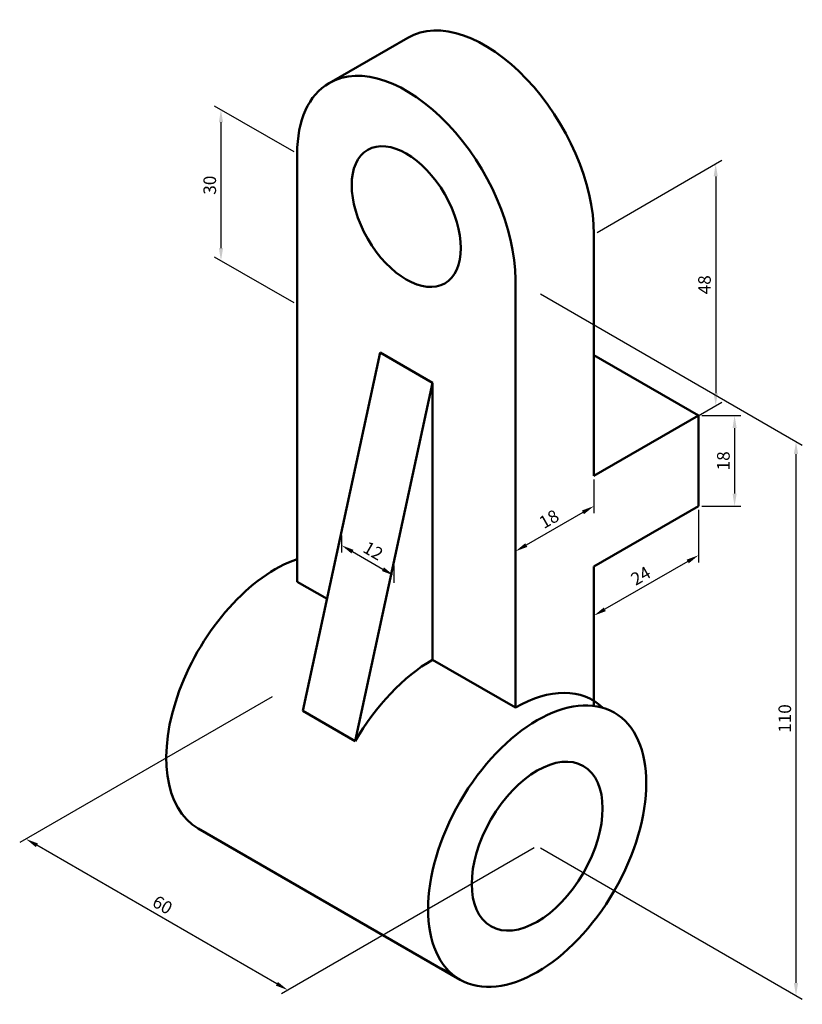
# Model space of a CAD drawing. Units: millimetres. Extents: x 3133 to 3289, y 1000 to 1195.
import ezdxf

# ---------------------------------------------------------------- set-up
doc = ezdxf.new("R2010")
doc.units = ezdxf.units.MM
doc.layers.add('M-DIMS', color=2, linetype='Continuous', lineweight=25)
doc.layers.add('M-OUTL', color=7, linetype='Continuous', lineweight=50)
doc.styles.get("Standard").update_dxf_attribs({"font": 'arial.ttf'})
doc.dimstyles.new('ISO-25', dxfattribs={"dimtxt": 2.5, "dimasz": 2.5, "dimexe": 1.25, "dimexo": 0.625, "dimtad": 1, "dimtxsty": 'Standard', "dimcen": 2.5, "dimadec": 0, "dimazin": 0, "dimtfac": 1, "dimtmove": 0, "dimatfit": 3, "dimfxl": 1, "dimarcsym": 0})

# ---------------------------------------------------------------- blocks, each defined once
blk = doc.blocks.new('*D1')
at = {"layer": 'Defpoints', "color": 0, "transparency": 16777216}
for p in [(3247.42, 1152.8), (3271.59, 1118.76), (3247.42, 1104.8)]:
    blk.add_point(p, dxfattribs=at)
at = {"layer": 'M-DIMS', "color": 0, "lineweight": -2, "transparency": 16777216}
for p, q in [((3248.04, 1153.16), (3272.84, 1167.48)), ((3271.59, 1164.26), (3271.59, 1121.26)), ((3248.04, 1105.16), (3272.84, 1119.48))]:
    blk.add_line(p, q, dxfattribs=at)
at = {"layer": 'M-DIMS', "color": 0, "transparency": 16777216}
for points in [[(3271.18, 1164.26), (3272.01, 1164.26), (3271.59, 1166.76)], [(3271.18, 1121.26), (3272.01, 1121.26), (3271.59, 1118.76)]]:
    blk.add_solid(points, dxfattribs=at)
at = {"layer": 'M-DIMS', "color": 0, "transparency": 16777216, "insert": (3269.69, 1142.76), "char_height": 2.5, "attachment_point": 5, "rotation": 90}
blk.add_mtext('48', dxfattribs=at)
blk = doc.blocks.new('*D2')
at = {"layer": 'Defpoints', "color": 0, "transparency": 16777216}
for p in [(3268.2, 1116.8), (3268.2, 1098.8), (3275.34, 1098.8)]:
    blk.add_point(p, dxfattribs=at)
at = {"layer": 'M-DIMS', "color": 0, "lineweight": -2, "transparency": 16777216}
for p, q in [((3268.83, 1116.8), (3276.59, 1116.8)), ((3275.34, 1114.3), (3275.34, 1101.3)), ((3268.83, 1098.8), (3276.59, 1098.8))]:
    blk.add_line(p, q, dxfattribs=at)
at = {"layer": 'M-DIMS', "color": 0, "transparency": 16777216}
for points in [[(3274.93, 1114.3), (3275.76, 1114.3), (3275.34, 1116.8)], [(3274.93, 1101.3), (3275.76, 1101.3), (3275.34, 1098.8)]]:
    blk.add_solid(points, dxfattribs=at)
at = {"layer": 'M-DIMS', "color": 0, "transparency": 16777216, "insert": (3273.44, 1107.8), "char_height": 2.5, "attachment_point": 5, "rotation": 90}
blk.add_mtext('18', dxfattribs=at)
blk = doc.blocks.new('*D3')
at = {"layer": 'Defpoints', "color": 0, "transparency": 16777216}
for p in [(3268.2, 1098.8), (3247.42, 1086.8), (3247.42, 1077.07)]:
    blk.add_point(p, dxfattribs=at)
at = {"layer": 'M-DIMS', "color": 0, "lineweight": -2, "transparency": 16777216}
for p, q in [((3268.2, 1098.08), (3268.2, 1087.62)), ((3266.04, 1087.82), (3249.58, 1078.32)), ((3247.42, 1086.08), (3247.42, 1075.62))]:
    blk.add_line(p, q, dxfattribs=at)
at = {"layer": 'M-DIMS', "color": 0, "transparency": 16777216}
for points in [[(3265.83, 1088.18), (3266.25, 1087.46), (3268.2, 1089.07)], [(3249.38, 1078.68), (3249.79, 1077.96), (3247.42, 1077.07)]]:
    blk.add_solid(points, dxfattribs=at)
at = {"layer": 'M-DIMS', "color": 0, "transparency": 16777216, "insert": (3256.87, 1084.7), "char_height": 2.5, "attachment_point": 5, "rotation": 30}
blk.add_mtext('24', dxfattribs=at)
blk = doc.blocks.new('*D4')
at = {"layer": 'Defpoints', "color": 0, "transparency": 16777216}
for p in [(3188.53, 1168.8), (3173.4, 1147.53), (3188.53, 1138.8)]:
    blk.add_point(p, dxfattribs=at)
at = {"layer": 'M-DIMS', "color": 0, "lineweight": -2, "transparency": 16777216}
for p, q in [((3187.9, 1169.16), (3172.15, 1178.25)), ((3173.4, 1175.03), (3173.4, 1150.03)), ((3187.9, 1139.16), (3172.15, 1148.25))]:
    blk.add_line(p, q, dxfattribs=at)
at = {"layer": 'M-DIMS', "color": 0, "transparency": 16777216}
for points in [[(3172.98, 1175.03), (3173.82, 1175.03), (3173.4, 1177.53)], [(3172.98, 1150.03), (3173.82, 1150.03), (3173.4, 1147.53)]]:
    blk.add_solid(points, dxfattribs=at)
at = {"layer": 'M-DIMS', "color": 0, "transparency": 16777216, "insert": (3171.5, 1162.53), "char_height": 2.5, "attachment_point": 5, "rotation": 90}
blk.add_mtext('30', dxfattribs=at)
blk = doc.blocks.new('*D5')
at = {"layer": 'Defpoints', "color": 0, "transparency": 16777216}
for p in [(3184.2, 1061.3), (3134.71, 1032.72), (3236.16, 1031.3)]:
    blk.add_point(p, dxfattribs=at)
at = {"layer": 'M-DIMS', "color": 0, "lineweight": -2, "transparency": 16777216}
for p, q in [((3183.57, 1060.94), (3133.46, 1032)), ((3184.5, 1003.97), (3136.87, 1031.47)), ((3235.54, 1030.94), (3185.42, 1002))]:
    blk.add_line(p, q, dxfattribs=at)
at = {"layer": 'M-DIMS', "color": 0, "transparency": 16777216}
for points in [[(3137.08, 1031.83), (3136.66, 1031.11), (3134.71, 1032.72)], [(3184.71, 1004.33), (3184.3, 1003.61), (3186.67, 1002.72)]]:
    blk.add_solid(points, dxfattribs=at)
at = {"layer": 'M-DIMS', "color": 0, "transparency": 16777216, "insert": (3161.64, 1019.37), "char_height": 2.5, "attachment_point": 5, "rotation": 330}
blk.add_mtext('60', dxfattribs=at)
blk = doc.blocks.new('*D6')
at = {"layer": 'Defpoints', "color": 0, "transparency": 16777216}
for p in [(3236.16, 1141.3), (3287.53, 1111.64), (3236.16, 1031.3)]:
    blk.add_point(p, dxfattribs=at)
at = {"layer": 'M-DIMS', "color": 0, "lineweight": -2, "transparency": 16777216}
for p, q in [((3236.79, 1140.94), (3288.78, 1110.92)), ((3287.53, 1004.14), (3287.53, 1109.14)), ((3236.79, 1030.94), (3288.78, 1000.92))]:
    blk.add_line(p, q, dxfattribs=at)
at = {"layer": 'M-DIMS', "color": 0, "transparency": 16777216}
for points in [[(3287.11, 1109.14), (3287.95, 1109.14), (3287.53, 1111.64)], [(3287.11, 1004.14), (3287.95, 1004.14), (3287.53, 1001.64)]]:
    blk.add_solid(points, dxfattribs=at)
at = {"layer": 'M-DIMS', "color": 0, "transparency": 16777216, "insert": (3285.63, 1056.64), "char_height": 2.5, "attachment_point": 5, "rotation": 90}
blk.add_mtext('110', dxfattribs=at)
blk = doc.blocks.new('*D7')
at = {"layer": 'Defpoints', "color": 0, "transparency": 16777216}
for p in [(3197.33, 1093.72), (3207.72, 1087.72), (3207.72, 1085.03)]:
    blk.add_point(p, dxfattribs=at)
at = {"layer": 'M-DIMS', "color": 0, "lineweight": -2, "transparency": 16777216}
for p, q in [((3197.33, 1093), (3197.33, 1089.58)), ((3199.49, 1089.78), (3205.56, 1086.28)), ((3207.72, 1087), (3207.72, 1083.58))]:
    blk.add_line(p, q, dxfattribs=at)
at = {"layer": 'M-DIMS', "color": 0, "transparency": 16777216}
for points in [[(3199.7, 1090.14), (3199.29, 1089.42), (3197.33, 1091.03)], [(3205.76, 1086.64), (3205.35, 1085.92), (3207.72, 1085.03)]]:
    blk.add_solid(points, dxfattribs=at)
at = {"layer": 'M-DIMS', "color": 0, "transparency": 16777216, "insert": (3203.46, 1089.66), "char_height": 2.5, "attachment_point": 5, "rotation": 330}
blk.add_mtext('12', dxfattribs=at)
blk = doc.blocks.new('*D8')
at = {"layer": 'Defpoints', "color": 0, "transparency": 16777216}
for p in [(3247.42, 1104.8), (3231.83, 1095.8), (3231.83, 1089.83)]:
    blk.add_point(p, dxfattribs=at)
at = {"layer": 'M-DIMS', "color": 0, "lineweight": -2, "transparency": 16777216}
for p, q in [((3247.42, 1104.08), (3247.42, 1097.38)), ((3245.25, 1097.57), (3233.99, 1091.08)), ((3231.83, 1095.08), (3231.83, 1088.38))]:
    blk.add_line(p, q, dxfattribs=at)
at = {"layer": 'M-DIMS', "color": 0, "transparency": 16777216}
for points in [[(3245.04, 1097.94), (3245.46, 1097.21), (3247.42, 1098.82)], [(3233.79, 1091.44), (3234.2, 1090.71), (3231.83, 1089.83)]]:
    blk.add_solid(points, dxfattribs=at)
at = {"layer": 'M-DIMS', "color": 0, "transparency": 16777216, "insert": (3238.67, 1095.97), "char_height": 2.5, "attachment_point": 5, "rotation": 29.9986}
blk.add_mtext('18', dxfattribs=at)

msp = doc.modelspace()

# ---------------------------------------------------------------- linework, layer by layer
at = {"layer": 'M-OUTL'}
for p, q in [((3210.458, 1191.814), (3194.87, 1182.814)), ((3188.529, 1168.798), (3188.529, 1083.798)), ((3247.418, 1152.798), (3247.418, 1104.798)), ((3231.83, 1143.798), (3231.83, 1058.798)), ((3189.674, 1058.136), (3204.983, 1129.298)), ((3215.375, 1123.298), (3204.983, 1129.298)), ((3268.203, 1116.798), (3247.418, 1128.798)), ((3215.375, 1123.298), (3200.066, 1052.136)), ((3215.375, 1123.298), (3215.375, 1068.298)), ((3247.418, 1104.798), (3268.203, 1116.798)), ((3268.203, 1116.798), (3268.203, 1098.798)), ((3268.203, 1098.798), (3247.418, 1086.798)), ((3247.418, 1086.798), (3247.418, 1059.152)), ((3194.458, 1080.374), (3188.529, 1083.798)), ((3215.375, 1068.298), (3231.83, 1058.798)), ((3200.066, 1052.136), (3189.674, 1058.136)), ((3168.889, 1034.781), (3220.851, 1004.781))]:
    msp.add_line(p, q, dxfattribs=at)
for centre, major_axis, start_param, end_param in [((3225.768, 1165.298), (15.309, -26.517), 7.0685835, 9.424778), ((3210.179, 1156.298), (15.309, -26.517), 0.7853982, 3.1415927), ((3210.179, 1156.298), (15.309, -26.517), 3.1415927, 3.9269908), ((3184.199, 1061.298), (-15.309, -26.517), 3.7256329, 6.2831853), ((3215.375, 1043.298), (-15.309, -26.517), 3.9269908, 4.712389), ((3231.83, 1033.798), (-15.309, -26.517), 2.9996956, 3.9269908), ((3231.83, 1033.798), (-15.309, -26.517), 0, 0.1418971)]:
    msp.add_ellipse(centre, major_axis=major_axis, ratio=0.5773503, start_param=start_param, end_param=end_param, dxfattribs=at)
for centre, major_axis in [((3210.179, 1156.298), (7.655, -13.258)), ((3236.16, 1031.298), (-15.309, -26.517)), ((3236.16, 1031.298), (-9.186, -15.91))]:
    msp.add_ellipse(centre, major_axis=major_axis, ratio=0.5773503, dxfattribs=at)

# ---------------------------------------------------------------- dimensions: what is measured, and where the dimension line sits
at = {"layer": 'M-DIMS'}
for p1, p2, distance, picture, middle in [((3188.529, 1168.798), (3188.529, 1138.798), -15.128, '*D4', (3171.499, 1162.532)), ((3247.418, 1152.798), (3247.418, 1104.798), 24.176, '*D1', (3269.693, 1142.756)), ((3236.16, 1031.298), (3236.16, 1141.298), -51.368, '*D6', (3285.627, 1056.64)), ((3268.203, 1116.798), (3268.203, 1098.798), 7.141, '*D2', (3273.443, 1107.798)), ((3247.418, 1104.798), (3231.83, 1095.798), 5.173, '*D8', (3238.673, 1095.972)), ((3268.203, 1098.798), (3247.418, 1086.798), 8.427, '*D3', (3256.871, 1084.696)), ((3197.328, 1093.717), (3207.721, 1087.717), -2.33, '*D7', (3203.465, 1089.655)), ((3236.16, 1031.298), (3184.199, 1061.298), 49.491, '*D5', (3161.639, 1019.371))]:
    dim = msp.add_aligned_dim(p1=p1, p2=p2, distance=distance, dimstyle='ISO-25', override={"dimclrd": 0, "dimclre": 0, "dimclrt": 0}, dxfattribs=at)
    dim.commit()
    dim.dimension.update_dxf_attribs({"geometry": picture, "text_midpoint": middle})

doc.saveas('drawing.dxf')
